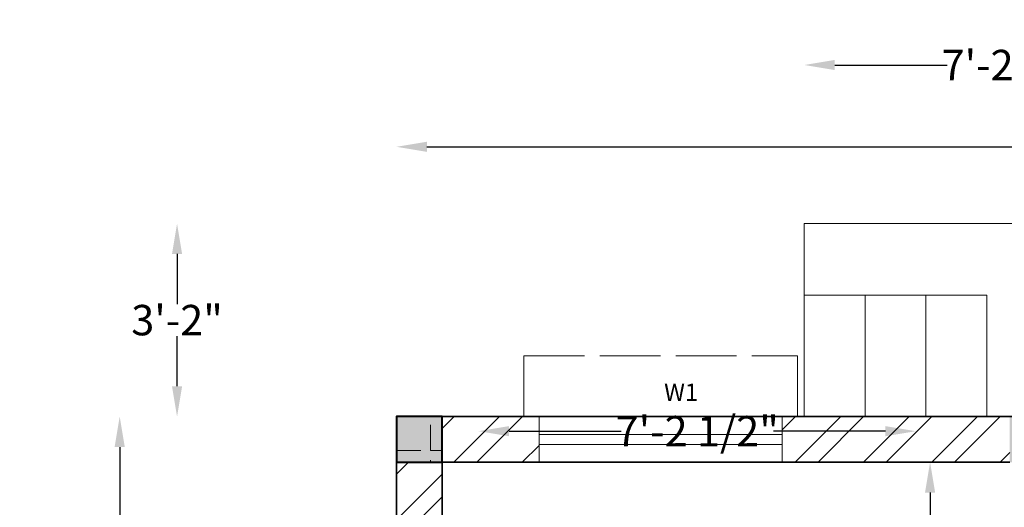
# Model space of a CAD drawing. Units: inches. Extents: x 3614 to 4242, y 2406 to 3033.
# Tile 6 of 10: x 3614 to 3808, y 2936 to 3033. Entities that reach past the tile are written whole.
import ezdxf

# ---------------------------------------------------------------- set-up
doc = ezdxf.new("R2010")
doc.units = ezdxf.units.IN
doc.linetypes.add('ACAD_ISO02W100', pattern=[15, 12, -3])
for name, color, linetype, lineweight in [('A-ANNO-DIMS', 2, 'Continuous', 18), ('A-ANNO-TEXT', 7, 'Continuous', 18), ('A-COLS', 7, 'Continuous', 40), ('A-COLS-PATT', 252, 'Continuous', 18), ('A-FLOR-STRS', 7, 'Continuous', 18), ('A-GLAZ', 4, 'Continuous', 18), ('A-GLAZ-OVHD', 8, 'ACAD_ISO02W100', 13), ('A-WALL', 7, 'Continuous', 35), ('A-WALL-PATT', 252, 'Continuous', 13)]:
    doc.layers.add(name, color=color, linetype=linetype, lineweight=lineweight)
doc.styles.get("Standard").update_dxf_attribs({"font": 'arial.ttf'})
doc.dimstyles.get("Standard").update_dxf_attribs({"dimtxt": 6, "dimasz": 6, "dimexe": 0.18, "dimexo": 0.0625, "dimgap": 0.09, "dimtad": 0, "dimtih": 1, "dimtoh": 1, "dimdec": 4, "dimzin": 0, "dimdsep": 46, "dimlunit": 4, "dimtxsty": 'Standard', "dimcen": 0.09, "dimse1": 1, "dimse2": 1, "dimadec": 0, "dimazin": 0, "dimtfac": 1, "dimtdec": 4, "dimtofl": 0, "dimtmove": 0, "dimatfit": 3, "dimfxl": 1, "dimtolj": 1, "dimtzin": 0, "dimarcsym": 0})

# ---------------------------------------------------------------- blocks, each defined once
blk = doc.blocks.new('*D15')
at = {"layer": 'A-ANNO-DIMS', "color": 0, "lineweight": -2, "transparency": 16777216}
for p, q in [((3793.63, 2939.34), (3793.63, 2846.99)), ((3793.63, 2748.34), (3793.63, 2840.69))]:
    blk.add_line(p, q, dxfattribs=at)
at = {"layer": 'A-ANNO-DIMS', "color": 0, "transparency": 16777216}
for points in [[(3792.63, 2939.34), (3794.63, 2939.34), (3793.63, 2945.34)], [(3792.63, 2748.34), (3794.63, 2748.34), (3793.63, 2742.34)]]:
    blk.add_solid(points, dxfattribs=at)
at = {"layer": 'Defpoints', "color": 0, "transparency": 16777216}
for p in [(3799.84, 2945.34), (3793.63, 2742.34), (3799.84, 2742.34)]:
    blk.add_point(p, dxfattribs=at)
at = {"layer": 'A-ANNO-DIMS', "color": 0, "transparency": 16777216, "insert": (3793.63, 2843.84), "char_height": 6, "attachment_point": 5}
blk.add_mtext('\\A1;16\'-11"', dxfattribs=at)
blk = doc.blocks.new('*D24')
at = {"layer": 'A-ANNO-DIMS', "color": 0, "lineweight": -2, "transparency": 16777216}
for p, q in [((3694.34, 3007.6), (3910.44, 3007.6)), ((4147.34, 3007.6), (3931.23, 3007.6))]:
    blk.add_line(p, q, dxfattribs=at)
at = {"layer": 'A-ANNO-DIMS', "color": 0, "transparency": 16777216}
for points in [[(3694.34, 3008.6), (3694.34, 3006.6), (3688.34, 3007.6)], [(4147.34, 3008.6), (4147.34, 3006.6), (4153.34, 3007.6)]]:
    blk.add_solid(points, dxfattribs=at)
at = {"layer": 'Defpoints', "color": 0, "transparency": 16777216}
for p in [(4153.34, 3007.6), (3688.34, 2954.34), (4153.34, 2954.34)]:
    blk.add_point(p, dxfattribs=at)
at = {"layer": 'A-ANNO-DIMS', "color": 0, "transparency": 16777216, "insert": (3920.84, 3007.6), "char_height": 6, "attachment_point": 5}
blk.add_mtext('\\A1;38\'-9"', dxfattribs=at)
blk = doc.blocks.new('*D26')
at = {"layer": 'A-ANNO-DIMS', "color": 0, "lineweight": -2, "transparency": 16777216}
for p, q in [((3633.72, 2948.34), (3633.72, 2707.46)), ((3633.72, 2452.14), (3633.72, 2693.02))]:
    blk.add_line(p, q, dxfattribs=at)
at = {"layer": 'A-ANNO-DIMS', "color": 0, "transparency": 16777216}
for points in [[(3632.72, 2948.34), (3634.72, 2948.34), (3633.72, 2954.34)], [(3632.72, 2452.14), (3634.72, 2452.14), (3633.72, 2446.14)]]:
    blk.add_solid(points, dxfattribs=at)
at = {"layer": 'Defpoints', "color": 0, "transparency": 16777216}
for p in [(3688.34, 2954.34), (3633.72, 2446.14), (3688.34, 2446.14)]:
    blk.add_point(p, dxfattribs=at)
at = {"layer": 'A-ANNO-DIMS', "color": 0, "transparency": 16777216, "insert": (3633.72, 2700.24), "char_height": 6, "attachment_point": 5}
blk.add_mtext('\\A1;42\'-4{\\H1x;\\S3/16;}"', dxfattribs=at)
blk = doc.blocks.new('WINDOW-W1-48IN')
for p, q in [((48, 9), (0, 9)), ((0, 9), (0, 0)), ((48, 0), (48, 9)), ((0, 5.5), (48, 5.5)), ((0, 3.5), (48, 3.5)), ((0, 0), (48, 0))]:
    blk.add_line(p, q)
blk = doc.blocks.new('SHADE-W1')
for p, q in [((0, 0), (0, 12)), ((0, 12), (51, 12)), ((51, 12), (54, 12)), ((54, 12), (54, 0)), ((3, 0), (0, 0))]:
    blk.add_line(p, q)
blk = doc.blocks.new('COLUMN-9X9')
blk.add_lwpolyline([(9, 9), (0, 9), (0, 0), (9, 0)], close=True)
blk = doc.blocks.new('*D64')
at = {"layer": 'A-ANNO-DIMS', "color": 0, "lineweight": -2, "transparency": 16777216}
for p, q in [((3710.55, 2951.47), (3732.66, 2951.47)), ((3784.82, 2951.47), (3762.72, 2951.47))]:
    blk.add_line(p, q, dxfattribs=at)
at = {"layer": 'A-ANNO-DIMS', "color": 0, "transparency": 16777216}
for points in [[(3710.55, 2952.47), (3710.55, 2950.47), (3704.55, 2951.47)], [(3784.82, 2952.47), (3784.82, 2950.47), (3790.82, 2951.47)]]:
    blk.add_solid(points, dxfattribs=at)
at = {"layer": 'Defpoints', "color": 0, "transparency": 16777216}
for p in [(3704.55, 2951.47), (3704.55, 2934.9), (3790.82, 2934.9)]:
    blk.add_point(p, dxfattribs=at)
at = {"layer": 'A-ANNO-DIMS', "color": 0, "transparency": 16777216, "insert": (3747.69, 2951.47), "char_height": 6, "attachment_point": 5}
blk.add_mtext('\\A1;7\'-2 1/2"', dxfattribs=at)
blk = doc.blocks.new('*D71')
at = {"layer": 'A-ANNO-DIMS', "color": 0, "lineweight": -2, "transparency": 16777216}
for p, q in [((3774.81, 3023.74), (3796.98, 3023.74)), ((3849.22, 3023.74), (3827.04, 3023.74))]:
    blk.add_line(p, q, dxfattribs=at)
at = {"layer": 'A-ANNO-DIMS', "color": 0, "transparency": 16777216}
for points in [[(3774.81, 3024.74), (3774.81, 3022.74), (3768.81, 3023.74)], [(3849.22, 3024.74), (3849.22, 3022.74), (3855.22, 3023.74)]]:
    blk.add_solid(points, dxfattribs=at)
at = {"layer": 'Defpoints', "color": 0, "transparency": 16777216}
for p in [(3855.22, 3023.74), (3768.81, 2992.44), (3855.22, 2992.44)]:
    blk.add_point(p, dxfattribs=at)
at = {"layer": 'A-ANNO-DIMS', "color": 0, "transparency": 16777216, "insert": (3812.01, 3023.74), "char_height": 6, "attachment_point": 5}
blk.add_mtext('\\A1;7\'-2 1/2"', dxfattribs=at)
blk = doc.blocks.new('*D72')
at = {"layer": 'A-ANNO-DIMS', "color": 0, "lineweight": -2, "transparency": 16777216}
for p, q in [((3645.04, 2986.44), (3645.04, 2976.54)), ((3645.04, 2960.34), (3645.04, 2970.23))]:
    blk.add_line(p, q, dxfattribs=at)
at = {"layer": 'A-ANNO-DIMS', "color": 0, "transparency": 16777216}
for points in [[(3644.04, 2986.44), (3646.04, 2986.44), (3645.04, 2992.44)], [(3644.04, 2960.34), (3646.04, 2960.34), (3645.04, 2954.34)]]:
    blk.add_solid(points, dxfattribs=at)
at = {"layer": 'Defpoints', "color": 0, "transparency": 16777216}
for p in [(3645.04, 2992.44), (3768.81, 2992.44), (3768.81, 2954.34)]:
    blk.add_point(p, dxfattribs=at)
at = {"layer": 'A-ANNO-DIMS', "color": 0, "transparency": 16777216, "insert": (3645.04, 2973.39), "char_height": 6, "attachment_point": 5}
blk.add_mtext('\\A1;3\'-2"', dxfattribs=at)

msp = doc.modelspace()

# ---------------------------------------------------------------- hatches: boundary and pattern name
at = {"layer": 'A-COLS-PATT'}
h = msp.add_hatch(dxfattribs=at)
h.set_pattern_fill('ANGLE', color=256)
h.set_pattern_definition([(0, (0, 0), (0, 6.985), [5.08, -1.905]), (90, (0, 0), (-6.985, 4e-16), [5.08, -1.905])])
h.paths.add_polyline_path([(3697.336, 2954.34049), (3688.336, 2954.34049), (3688.336, 2945.34049), (3697.336, 2945.34049)])
h = msp.add_hatch(color=256, dxfattribs=at)
h.dxf.hatch_style = 1
h.paths.add_polyline_path([(3697.336, 2954.34049), (3688.336, 2954.34049), (3688.336, 2945.34049), (3697.336, 2945.34049)])
h.paths.add_polyline_path([(3818.336, 2954.34049), (3809.336, 2954.34049), (3809.336, 2945.34049), (3818.336, 2945.34049)])
h.paths.add_polyline_path([(3818.336, 2787.28572), (3809.336, 2787.28572), (3809.336, 2778.34049), (3818.336, 2778.34049)])
h.paths.add_polyline_path([(3697.336, 2742.34049), (3688.336, 2742.34049), (3688.336, 2733.34049), (3697.336, 2733.34049)])
h.paths.add_polyline_path([(3697.336, 2583.37355), (3688.336, 2583.37355), (3688.336, 2574.37355), (3697.336, 2574.37355)])
h.paths.add_polyline_path([(3899.336, 2583.34049), (3890.336, 2583.34049), (3890.336, 2574.34049), (3899.336, 2574.34049)])
h.paths.add_polyline_path([(3983.336, 2583.34049), (3974.336, 2583.34049), (3974.336, 2574.34049), (3983.336, 2574.34049)])
h.paths.add_polyline_path([(4153.336, 2583.34049), (4144.336, 2583.34049), (4144.336, 2574.34049), (4153.336, 2574.34049)])
h.paths.add_polyline_path([(4153.336, 2742.34049), (4144.336, 2742.34049), (4144.336, 2733.34049), (4153.336, 2733.34049)])
h.paths.add_polyline_path([(4153.336, 2795.34049), (4144.336, 2795.34049), (4144.336, 2786.34049), (4153.336, 2786.34049)])
h.paths.add_polyline_path([(3983.336, 2795.31105), (3974.336, 2795.31105), (3974.336, 2786.34049), (3983.336, 2786.34049)])
h.paths.add_polyline_path([(4153.336, 2954.34049), (4144.36882, 2954.34049), (4144.36882, 2945.34049), (4153.336, 2945.34049)])
h.paths.add_polyline_path([(3982.96188, 2954.34049), (3973.96188, 2954.34049), (3973.96188, 2945.34049), (3982.96188, 2945.34049)])
at = {"layer": 'A-WALL-PATT'}
h = msp.add_hatch(dxfattribs=at)
h.set_pattern_fill('ANSI32', color=256)
h.paths.add_polyline_path([(4041.01458, 2954.34049), (3982.96188, 2954.34049), (3982.96188, 2945.34049), (3983.336, 2945.34049), (4041.01458, 2945.34049)])
h.paths.add_polyline_path([(3973.96188, 2954.34049), (3960.11861, 2954.34049), (3960.11861, 2945.34049), (3973.96188, 2945.34049)])
h.paths.add_polyline_path([(3936.11861, 2954.34049), (3901.17016, 2954.34049), (3901.17016, 2945.34049), (3913.336, 2945.34049), (3913.336, 2896.34049, -0.050382044), (3919.336, 2895.73437), (3919.336, 2945.34049), (3936.11861, 2945.34049)])
h.paths.add_polyline_path([(3983.336, 2945.34049), (3982.96188, 2945.34049), (3974.336, 2945.34049), (3974.336, 2873.34049), (3974.336, 2795.31105), (3983.336, 2795.31105), (3983.336, 2867.34049)])
h.paths.add_polyline_path([(3974.336, 2872.34049), (3919.336, 2872.34049), (3858.336, 2872.34049), (3858.336, 2866.34049), (3919.336, 2866.34049), (3974.336, 2866.34049)])
h.paths.add_polyline_path([(3877.17016, 2954.34049), (3852.34021, 2954.34049), (3852.34021, 2945.34049), (3852.336, 2896.34049), (3858.336, 2896.34049), (3858.336, 2945.34049), (3877.17016, 2945.34049)])
h.paths.add_polyline_path([(3871.94212, 2902.34049), (3858.336, 2902.34049), (3858.336, 2896.34049), (3871.336, 2896.34049, -0.050382044)], flags=0)
h.paths.add_polyline_path([(3913.336, 2902.34049), (3901.336, 2902.34049), (3901.336, 2896.34049), (3913.336, 2896.34049)], flags=17)
h.paths.add_polyline_path([(3858.336, 2872.34049), (3852.336, 2872.34049), (3852.336, 2866.34049), (3858.336, 2866.34049)])
h.paths.add_polyline_path([(3809.336, 2954.34049), (3764.4617, 2954.34049), (3764.4617, 2945.34049), (3809.336, 2945.34049)])
h.paths.add_polyline_path([(3716.4617, 2954.34049), (3697.336, 2954.34049), (3697.336, 2945.34049), (3716.4617, 2945.34049)])
h.paths.add_polyline_path([(3697.336, 2945.34049), (3688.336, 2945.34049), (3688.336, 2894.73438), (3697.336, 2894.73438)])

# ---------------------------------------------------------------- linework, layer by layer
at = {"layer": 'A-FLOR-STRS'}
for p, q in [((3768.80751, 2954.34049), (3768.80751, 2992.43626)), ((3768.80751, 2992.43626), (3855.21729, 2992.43626)), ((3780.80751, 2978.34049), (3768.80751, 2978.34049)), ((3768.80751, 2978.34049), (3768.80751, 2954.34049)), ((3780.80751, 2954.34049), (3780.80751, 2978.34049)), ((3780.80751, 2978.34049), (3804.80751, 2978.34049)), ((3792.80751, 2954.34049), (3792.80751, 2978.34049)), ((3804.80751, 2978.34049), (3792.80751, 2978.34049)), ((3804.80751, 2954.34049), (3804.80751, 2978.34049))]:
    msp.add_line(p, q, dxfattribs=at)
at = {"layer": 'A-WALL'}
for p, q in [((3688.336, 2954.34049), (3688.336, 2574.34049)), ((3688.336, 2954.34049), (3820.48336, 2954.34049)), ((3697.336, 2945.34049), (3697.336, 2742.34049)), ((3697.336, 2945.34049), (3809.336, 2945.34049))]:
    msp.add_line(p, q, dxfattribs=at)

# ---------------------------------------------------------------- block references
at = {"layer": 'A-COLS'}
msp.add_blockref('COLUMN-9X9', (3688.336, 2945.34), dxfattribs=at)
at = {"layer": 'A-GLAZ'}
msp.add_blockref('WINDOW-W1-48IN', (3716.462, 2945.34), dxfattribs=at)
at = {"layer": 'A-GLAZ-OVHD'}
msp.add_blockref('SHADE-W1', (3713.462, 2954.34), dxfattribs=at)

# ---------------------------------------------------------------- texts
at = {"layer": 'A-ANNO-TEXT', "insert": (3741.14695, 2960.86625), "char_height": 3.42604, "attachment_point": 1}
msp.add_mtext_dynamic_manual_height_columns('W1', width=192.8287007, gutter_width=17.1302, heights=[0], dxfattribs=at)

# ---------------------------------------------------------------- dimensions: what is measured, and where the dimension line sits
at = {"layer": 'A-ANNO-DIMS'}
for base, p1, p2, override, picture, middle in [((3855.21729, 3023.73626), (3768.80751, 2992.43626), (3855.21729, 2992.43626), {"dimdec": 1, "dimlfac": 1, "dimrnd": 0, "dimzin": 1, "dimdsep": 46, "dimlunit": 4, "dimfrac": 2}, '*D71', (3812.0124, 3023.73626)), ((4153.336, 3007.59551), (3688.336, 2954.34049), (4153.336, 2954.34049), {"dimclrd": 0, "dimclre": 0, "dimclrt": 0}, '*D24', (3920.836, 3007.59551))]:
    dim = msp.add_linear_dim(base=base, p1=p1, p2=p2, dimstyle='Standard', override=override, dxfattribs=at)
    dim.commit()
    dim.dimension.update_dxf_attribs({"geometry": picture, "text_midpoint": middle})
for base, p1, p2, angle, override, picture, middle in [((3645.036, 2992.43626), (3768.80751, 2954.34049), (3768.80751, 2992.43626), 90, {"dimdec": 1, "dimlfac": 1, "dimrnd": 0, "dimzin": 1, "dimdsep": 46, "dimlunit": 4, "dimfrac": 2}, '*D72', (3645.036, 2973.38838)), ((3704.5532, 2951.4657), (3790.82041, 2934.90029), (3704.5532, 2934.90029), 180, {"dimdec": 1, "dimlfac": 1, "dimrnd": 0, "dimzin": 1, "dimdsep": 46, "dimlunit": 4, "dimfrac": 2}, '*D64', (3747.68681, 2951.4657)), ((3633.71834, 2446.14049), (3688.336, 2954.34049), (3688.336, 2446.14049), 90, {"dimclrd": 0, "dimclre": 0, "dimclrt": 0}, '*D26', (3633.71834, 2700.24049)), ((3793.63235, 2742.34049), (3799.84322, 2945.34049), (3799.84322, 2742.34049), 90, {"dimclrd": 0, "dimclre": 0, "dimclrt": 0}, '*D15', (3793.63235, 2843.84049))]:
    dim = msp.add_linear_dim(base=base, p1=p1, p2=p2, angle=angle, dimstyle='Standard', override=override, dxfattribs=at)
    dim.commit()
    dim.dimension.update_dxf_attribs({"geometry": picture, "text_midpoint": middle})

doc.saveas('drawing.dxf')
